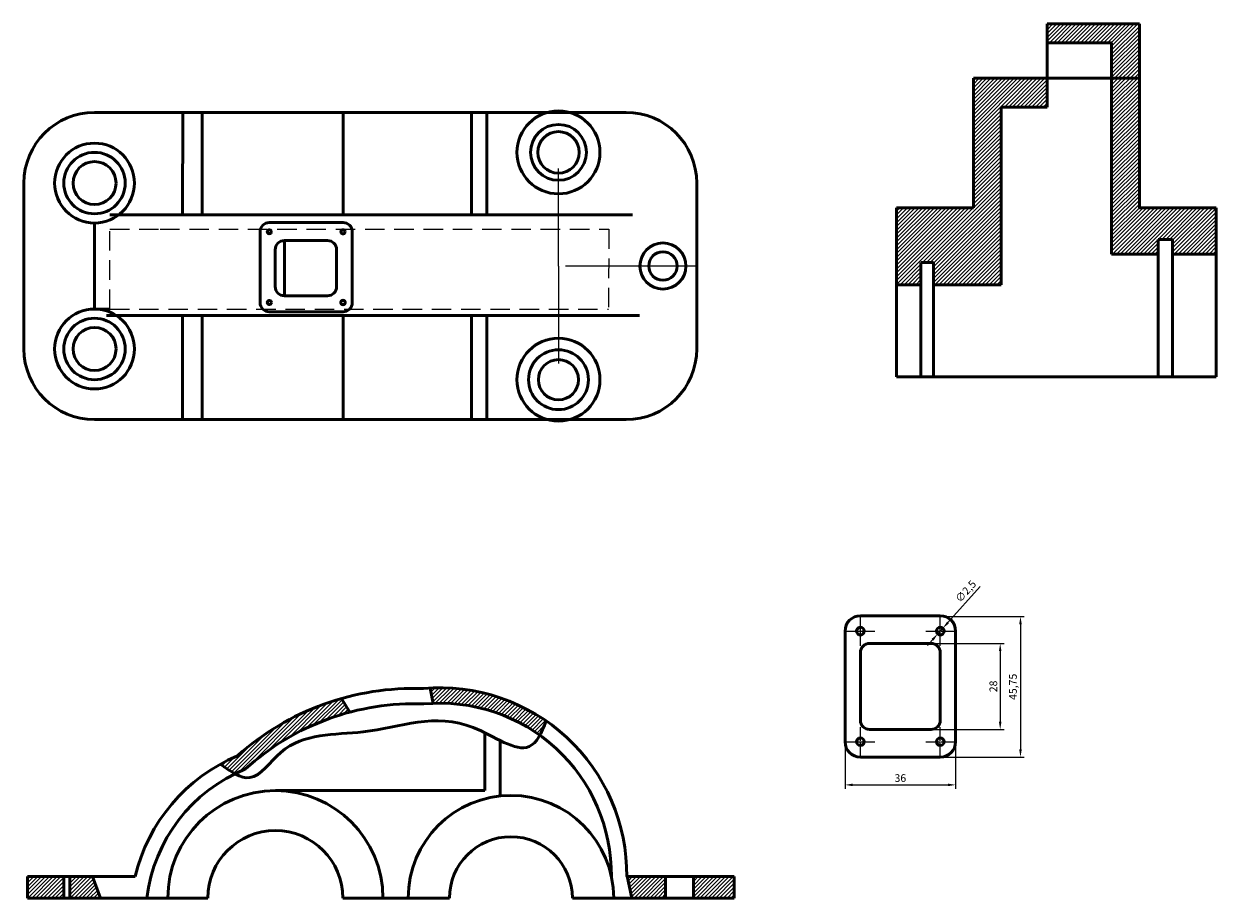
# Model space of a CAD drawing. Units: millimetres. Extents: x 982 to 1370, y 1632 to 1917.
import ezdxf

# ---------------------------------------------------------------- set-up
doc = ezdxf.new("R2010")
doc.units = ezdxf.units.MM
doc.linetypes.add('CENTER', pattern=[50.800000000000004, 31.75, -6.349999999999999, 6.349999999999999, -6.349999999999999])
doc.linetypes.add('HIDDEN', pattern=[9.524999999999999, 6.349999999999999, -3.174999999999999])
for name, color, linetype, lineweight in [('M-CNTR', 1, 'CENTER', 18), ('M-DIMS', 2, 'Continuous', 25), ('M-HATC', 8, 'Continuous', 18), ('M-HIDN', 6, 'HIDDEN', 25), ('M-OUTL', 7, 'Continuous', 50)]:
    doc.layers.add(name, color=color, linetype=linetype, lineweight=lineweight)
doc.styles.get("Standard").update_dxf_attribs({"font": 'arial.ttf'})
doc.dimstyles.new('ISO-25', dxfattribs={"dimtxt": 2.5, "dimasz": 2.5, "dimexe": 1.25, "dimexo": 0.625, "dimtad": 1, "dimtxsty": 'Standard', "dimcen": 2.5, "dimadec": 0, "dimazin": 0, "dimtfac": 1, "dimtmove": 0, "dimatfit": 3, "dimfxl": 1, "dimarcsym": 0})
pattern_1 = [(45, (0, 0), (-0.6286179284748407, 0.6286179284748407), [])]

# ---------------------------------------------------------------- blocks, each defined once
blk = doc.blocks.new('*U1')
at = {"layer": 'M-CNTR', "color": 0, "transparency": 16777216}
for p, q in [((0, 0.25), (0, 4.75)), ((-4.75, 0), (-0.25, 0)), ((0.25, 0), (4.75, 0)), ((0, -4.75), (0, -0.25))]:
    blk.add_line(p, q, dxfattribs=at)
at = {"layer": 'M-CNTR', "color": 0, "linetype": 'Continuous', "transparency": 16777216}
for p, q in [((-0.125, 0), (0.125, 0)), ((0, -0.125), (0, 0.125))]:
    blk.add_line(p, q, dxfattribs=at)
blk = doc.blocks.new('*U2')
at = {"layer": 'M-CNTR', "color": 0, "transparency": 16777216}
for p, q in [((0, 0.25), (0, 4.75)), ((-4.75, 0), (-0.25, 0)), ((0.25, 0), (4.75, 0)), ((0, -4.75), (0, -0.25))]:
    blk.add_line(p, q, dxfattribs=at)
at = {"layer": 'M-CNTR', "color": 0, "linetype": 'Continuous', "transparency": 16777216}
for p, q in [((-0.125, 0), (0.125, 0)), ((0, -0.125), (0, 0.125))]:
    blk.add_line(p, q, dxfattribs=at)
blk = doc.blocks.new('*U3')
at = {"layer": 'M-CNTR', "color": 0, "transparency": 16777216}
for p, q in [((0, 0.25), (0, 4.75)), ((-4.75, 0), (-0.25, 0)), ((0.25, 0), (4.75, 0)), ((0, -4.75), (0, -0.25))]:
    blk.add_line(p, q, dxfattribs=at)
at = {"layer": 'M-CNTR', "color": 0, "linetype": 'Continuous', "transparency": 16777216}
for p, q in [((-0.125, 0), (0.125, 0)), ((0, -0.125), (0, 0.125))]:
    blk.add_line(p, q, dxfattribs=at)
blk = doc.blocks.new('*U4')
at = {"layer": 'M-CNTR', "color": 0, "transparency": 16777216}
for p, q in [((0, 0.25), (0, 4.75)), ((-4.75, 0), (-0.25, 0)), ((0.25, 0), (4.75, 0)), ((0, -4.75), (0, -0.25))]:
    blk.add_line(p, q, dxfattribs=at)
at = {"layer": 'M-CNTR', "color": 0, "linetype": 'Continuous', "transparency": 16777216}
for p, q in [((-0.125, 0), (0.125, 0)), ((0, -0.125), (0, 0.125))]:
    blk.add_line(p, q, dxfattribs=at)
blk = doc.blocks.new('*D5')
at = {"layer": 'Defpoints', "color": 0, "transparency": 16777216}
for p in [(1249.511989077973, 1683.208601525211), (1285.511989077973, 1683.208601525211), (1285.511989077973, 1669.151294933958)]:
    blk.add_point(p, dxfattribs=at)
at = {"layer": 'M-DIMS', "color": 0, "lineweight": -2, "transparency": 16777216}
for p, q in [((1249.511989077973, 1682.583601525211), (1249.511989077973, 1667.901294933958)), ((1285.511989077973, 1682.583601525211), (1285.511989077973, 1667.901294933958)), ((1252.011989077973, 1669.151294933958), (1283.011989077973, 1669.151294933958))]:
    blk.add_line(p, q, dxfattribs=at)
at = {"layer": 'M-DIMS', "color": 0, "transparency": 16777216}
for points in [[(1252.011989077973, 1669.567961600625), (1252.011989077973, 1668.734628267292), (1249.511989077973, 1669.151294933958)], [(1283.011989077973, 1669.567961600625), (1283.011989077973, 1668.734628267292), (1285.511989077973, 1669.151294933958)]]:
    blk.add_solid(points, dxfattribs=at)
at = {"layer": 'M-DIMS', "color": 0, "transparency": 16777216, "insert": (1267.511989077973, 1671.053580063563), "char_height": 2.5, "attachment_point": 5}
blk.add_mtext('36', dxfattribs=at)
blk = doc.blocks.new('*D6')
at = {"layer": 'Defpoints', "color": 0, "transparency": 16777216}
for p in [(1280.511989077974, 1723.958601525212), (1280.511989077974, 1678.208601525212), (1306.611679596875, 1678.208601525212)]:
    blk.add_point(p, dxfattribs=at)
at = {"layer": 'M-DIMS', "color": 0, "lineweight": -2, "transparency": 16777216}
for p, q in [((1281.136989077974, 1723.958601525212), (1307.861679596875, 1723.958601525212)), ((1306.611679596875, 1721.458601525213), (1306.611679596875, 1680.708601525212)), ((1281.136989077974, 1678.208601525212), (1307.861679596875, 1678.208601525212))]:
    blk.add_line(p, q, dxfattribs=at)
at = {"layer": 'M-DIMS', "color": 0, "transparency": 16777216}
for points in [[(1306.195012930208, 1721.458601525213), (1307.028346263542, 1721.458601525213), (1306.611679596875, 1723.958601525212)], [(1306.195012930208, 1680.708601525212), (1307.028346263542, 1680.708601525212), (1306.611679596875, 1678.208601525212)]]:
    blk.add_solid(points, dxfattribs=at)
at = {"layer": 'M-DIMS', "color": 0, "transparency": 16777216, "insert": (1304.489408109836, 1701.083601525211), "char_height": 2.5, "attachment_point": 5, "rotation": 90}
blk.add_mtext('45,75', dxfattribs=at)
blk = doc.blocks.new('*D7')
at = {"layer": 'Defpoints', "color": 0, "transparency": 16777216}
for p in [(1277.511989077974, 1715.208601525213), (1277.511989077974, 1687.208601525212), (1300.009759810087, 1687.208601525212)]:
    blk.add_point(p, dxfattribs=at)
at = {"layer": 'M-DIMS', "color": 0, "lineweight": -2, "transparency": 16777216}
for p, q in [((1278.136989077974, 1715.208601525213), (1301.259759810087, 1715.208601525213)), ((1300.009759810087, 1712.708601525212), (1300.009759810087, 1689.708601525212)), ((1278.136989077974, 1687.208601525212), (1301.259759810087, 1687.208601525212))]:
    blk.add_line(p, q, dxfattribs=at)
at = {"layer": 'M-DIMS', "color": 0, "transparency": 16777216}
for points in [[(1299.59309314342, 1712.708601525212), (1300.426426476754, 1712.708601525212), (1300.009759810087, 1715.208601525213)], [(1299.59309314342, 1689.708601525212), (1300.426426476754, 1689.708601525212), (1300.009759810087, 1687.208601525212)]]:
    blk.add_solid(points, dxfattribs=at)
at = {"layer": 'M-DIMS', "color": 0, "transparency": 16777216, "insert": (1298.108327340783, 1701.208601525212), "char_height": 2.5, "attachment_point": 5, "rotation": 90}
blk.add_mtext('28', dxfattribs=at)
blk = doc.blocks.new('*D8')
at = {"layer": 'Defpoints', "color": 0, "transparency": 16777216}
for p in [(1281.346385037726, 1720.139344981997), (1279.677593118221, 1718.277858068427)]:
    blk.add_point(p, dxfattribs=at)
at = {"layer": 'M-DIMS', "color": 0, "lineweight": -2, "transparency": 16777216}
for p, q in [((1293.494623055285, 1733.690337066936), (1283.015176957231, 1722.000831895568)), ((1279.677593118221, 1718.277858068427), (1281.346385037726, 1720.139344981997)), ((1278.008801198716, 1716.416371154856), (1276.34000927921, 1714.554884241286))]:
    blk.add_line(p, q, dxfattribs=at)
at = {"layer": 'M-DIMS', "color": 0, "transparency": 16777216}
for points in [[(1282.704929138303, 1722.278963882152), (1283.32542477616, 1721.722699908983), (1281.346385037726, 1720.139344981997)], [(1277.698553379787, 1716.69450314144), (1278.319049017644, 1716.138239168272), (1279.677593118221, 1718.277858068427)]]:
    blk.add_solid(points, dxfattribs=at)
at = {"layer": 'M-DIMS', "color": 0, "transparency": 16777216, "insert": (1289.029728391543, 1731.958212710914), "char_height": 2.5, "attachment_point": 5, "rotation": 48.12430414894632}
blk.add_mtext('∅2,5', dxfattribs=at)

msp = doc.modelspace()

# ---------------------------------------------------------------- hatches: boundary and pattern name
at = {"layer": 'M-HATC'}
h = msp.add_hatch(dxfattribs=at)
h.set_pattern_fill('ANSI31', color=256, scale=0.28)
h.set_pattern_definition(pattern_1)
h.paths.add_polyline_path([(1300.29876673081, 1889.791887260162), (1315.29876673081, 1889.791887260162), (1315.29876673081, 1899.183957242303), (1291.29876673081, 1899.183957242303), (1291.29876673081, 1856.97244571802), (1266.29876673081, 1856.97244571802), (1266.29876673081, 1831.97244571802), (1274.206576974626, 1831.97244571802), (1274.206576974626, 1839.244321779904), (1278.280369147082, 1839.244321779905), (1278.280369147082, 1831.97244571802), (1300.29876673081, 1831.97244571802)])
h.paths.add_polyline_path([(1370.29876673081, 1856.97244571802), (1345.29876673081, 1856.97244571802), (1345.29876673081, 1899.183957242303), (1336.285268659707, 1899.183957242303), (1336.285268659707, 1841.97244571802), (1351.382184464795, 1841.97244571802), (1351.382184464795, 1846.706406237832), (1356.134930561908, 1846.706406237832), (1356.134930561908, 1841.97244571802), (1370.29876673081, 1841.97244571802)])
h.paths.add_polyline_path([(1345.29876673081, 1916.899596030982), (1340.29876673081, 1916.899596030982), (1315.29876673081, 1916.899596030982), (1315.29876673081, 1910.726026523388), (1336.285268659707, 1910.726026523388), (1336.285268659707, 1899.183957242303), (1345.29876673081, 1899.183957242303)])
h = msp.add_hatch(dxfattribs=at)
h.set_pattern_fill('ANSI31', color=256, scale=0.28)
h.set_pattern_definition(pattern_1)
h.paths.add_polyline_path([(995.2535490241661, 1639.282014954298), (983.4732738171352, 1639.282014954298), (983.4732738171352, 1632.282014954298), (995.2535490241661, 1632.282014954298)])
h.paths.add_polyline_path([(1004.648487103659, 1639.282014954298), (997.2535490241662, 1639.282014954298), (997.2535490241662, 1632.282014954298), (1007.250709303537, 1632.282014954298)])
edge = h.paths.add_edge_path()
edge.add_line((1088.387454769102, 1692.837831887581), (1085.605211651708, 1697.258198737764))
edge.add_arc((1109.271975537356, 1614.115057323262), 86.44592342667784, 105.8890469631471, 131.7276792270625)
edge.add_arc((1074.062003103345, 1626.025891843346), 57.14745509284148, 112.9982183834284, 119.206106940538)
edge.add_spline(control_points=[(1046.176748216584, 1675.908195153124), (1047.783063834055, 1674.759506472575), (1049.389379451526, 1673.610817792025), (1050.94946138008, 1672.771666922494)], knot_values=[0, 0, 0, 0, 5.081182044010842, 5.081182044010842, 5.081182044010842, 5.081182044010842], degree=3, periodic=0)
edge.add_arc((1074.062003103346, 1626.025891843347), 52.14745509284142, 112.09848204372611, 116.30920051008201, ccw=False)
edge.add_arc((1109.271975537356, 1614.115057323262), 81.44592342667777, 104.8578574495586, 132.313036151602, ccw=False)
edge = h.paths.add_edge_path()
edge.add_line((1114.536751154887, 1700.664583068479), (1115.499488170572, 1695.703224651357))
edge.add_arc((1117.676663324449, 1639.945484012596), 55.80023058007832, 54.3761729250636, 92.23609505560682, ccw=False)
edge.add_spline(control_points=[(1150.178124588469, 1685.303181799117), (1150.925335073614, 1686.661176424872), (1151.580506534144, 1688.273325651683), (1152.195395815112, 1689.996709230653)], knot_values=[112.2880017170733, 112.2880017170733, 112.2880017170733, 112.2880017170733, 116.9515328515951, 116.9515328515951, 116.9515328515951, 116.9515328515951], degree=3, periodic=0)
edge.add_arc((1117.676663324449, 1639.945484012596), 60.80023058007828, 55.40721006559874, 92.96024829593541)
h.paths.add_polyline_path([(1191.134183879782, 1639.282014954298), (1178.620543520746, 1639.282014954298), (1180.136133887702, 1632.282014954298), (1191.134183879781, 1632.282014954298)])
h.paths.add_polyline_path([(1213.473273817135, 1639.282014954298), (1200.175070862797, 1639.282014954298), (1200.175070862797, 1632.282014954298), (1213.473273817135, 1632.282014954298)])

# ---------------------------------------------------------------- linework, layer by layer
at = {"layer": 'M-CNTR'}
for p, q in [((1156.251070972097, 1838.057992080775), (1156.251070972097, 1875.057992080776)), ((1190.251070972097, 1838.057992080775), (1156.251070972097, 1838.057992080775)), ((1156.251070972097, 1838.057992080775), (1156.251070972097, 1801.057992080776)), ((1201.251070972097, 1838.057992080775), (1190.251070972097, 1838.057992080775))]:
    msp.add_line(p, q, dxfattribs=at)
at = {"layer": 'M-HIDN'}
for p, q in [((1010.251070972097, 1824.057992080776), (1010.251070972097, 1850.036021916558)), ((1010.251070972097, 1850.036021916558), (1026.612848150797, 1850.036021916558)), ((1026.612848150797, 1850.036021916558), (1172.670257073025, 1850.036021916558)), ((1172.670257073025, 1850.036021916558), (1172.528142112141, 1824.057992080776)), ((1010.251070972097, 1824.057992080776), (1172.528142112141, 1824.057992080776))]:
    msp.add_line(p, q, dxfattribs=at)
at = {"layer": 'M-OUTL'}
for p, q in [((1315.29876673081, 1889.791887260162), (1315.29876673081, 1916.899596030982)), ((1315.29876673081, 1916.899596030982), (1340.29876673081, 1916.899596030982)), ((1340.29876673081, 1916.899596030982), (1345.29876673081, 1916.899596030982)), ((1345.29876673081, 1916.899596030982), (1345.29876673081, 1899.183957242303)), ((1336.285268659707, 1910.726026523388), (1315.29876673081, 1910.726026523388)), ((1336.285268659707, 1841.97244571802), (1336.285268659707, 1910.726026523388)), ((1291.29876673081, 1856.97244571802), (1291.29876673081, 1899.183957242303)), ((1291.29876673081, 1899.183957242303), (1345.29876673081, 1899.183957242303)), ((1345.29876673081, 1856.97244571802), (1345.29876673081, 1899.183957242303)), ((1005.251070972097, 1888.057992080776), (1178.251070972097, 1888.057992080776)), ((1034.029285878291, 1888.057992080776), (1033.904053084971, 1854.694341917483)), ((1040.294262971387, 1888.057992080776), (1040.294262971387, 1854.694341917483)), ((1086.162194136173, 1888.057992080776), (1086.162194136173, 1854.694341917483)), ((1127.916033374389, 1888.057992080776), (1127.916033374389, 1854.694341917483)), ((1132.916033374389, 1854.694341917483), (1132.916033374389, 1888.057992080776)), ((1300.29876673081, 1831.97244571802), (1300.29876673081, 1889.791887260162)), ((1300.29876673081, 1889.791887260162), (1315.29876673081, 1889.791887260162)), ((982.2510709720972, 1811.057992080776), (982.2510709720972, 1865.057992080776)), ((1201.251070972097, 1811.057992080776), (1201.251070972097, 1865.057992080776)), ((1266.29876673081, 1801.97244571802), (1266.29876673081, 1856.97244571802)), ((1266.29876673081, 1856.97244571802), (1291.29876673081, 1856.97244571802)), ((1266.29876673081, 1856.97244571802), (1266.29876673081, 1831.97244571802)), ((1370.29876673081, 1856.97244571802), (1345.29876673081, 1856.97244571802)), ((1370.29876673081, 1801.97244571802), (1370.29876673081, 1856.97244571802)), ((1370.29876673081, 1856.97244571802), (1370.29876673081, 1841.97244571802)), ((1005.251070972097, 1852.057992080776), (1005.251070972097, 1824.057992080776)), ((1010.252314597974, 1854.694341917483), (1180.329749461996, 1854.694341917483)), ((1062.143259161312, 1852.211589826624), (1086.143259161312, 1852.211589826624)), ((1059.143259161312, 1849.211589826624), (1059.143259161312, 1826.179334016416)), ((1089.143259161312, 1826.179334016416), (1089.143259161312, 1849.211589826624)), ((1064.050993755085, 1831.375096835255), (1064.050993755085, 1843.375096835255)), ((1067.050993755085, 1846.375096835255), (1081.050993755085, 1846.375096835255)), ((1067.050993755085, 1846.375096835255), (1067.050993755085, 1828.375096835255)), ((1084.050993755085, 1843.375096835255), (1084.050993755085, 1831.375096835255)), ((1351.382184464795, 1846.706406237832), (1351.382184464795, 1801.97244571802)), ((1351.382184464795, 1846.706406237832), (1356.134930561908, 1846.706406237832)), ((1356.134930561908, 1801.97244571802), (1356.134930561908, 1846.706406237832)), ((1351.382184464795, 1841.97244571802), (1336.285268659707, 1841.97244571802)), ((1370.29876673081, 1841.97244571802), (1356.134930561908, 1841.97244571802)), ((1274.206576974626, 1839.244321779904), (1274.206576974626, 1801.97244571802)), ((1274.206576974626, 1839.244321779904), (1278.280369147082, 1839.244321779905)), ((1278.280369147082, 1801.97244571802), (1278.280369147082, 1839.244321779905)), ((1266.29876673081, 1831.97244571802), (1274.206576974626, 1831.97244571802)), ((1278.280369147082, 1831.97244571802), (1300.29876673081, 1831.97244571802)), ((1081.050993755085, 1828.375096835255), (1067.050993755085, 1828.375096835255)), ((1005.251070972097, 1824.057992080776), (1010.251070972097, 1824.057992080776)), ((1009.203594559912, 1821.924287656346), (1182.625737453978, 1821.924287656346)), ((1033.904053084971, 1821.924287656345), (1033.904053084971, 1788.057992080776)), ((1040.294262971387, 1821.924287656346), (1040.294262971387, 1788.057992080776)), ((1062.143259161312, 1823.179334016416), (1086.143259161312, 1823.179334016416)), ((1086.162194136173, 1821.924287656346), (1086.162194136173, 1788.057992080776)), ((1127.916033374389, 1821.924287656345), (1127.916033374389, 1788.057992080776)), ((1132.916033374389, 1821.924287656345), (1132.916033374389, 1788.057992080776)), ((1266.29876673081, 1801.97244571802), (1370.29876673081, 1801.97244571802)), ((1005.251070972097, 1788.057992080776), (1178.251070972097, 1788.057992080776)), ((1254.511989077973, 1724.208601525212), (1280.511989077973, 1724.208601525212)), ((1249.511989077973, 1683.208601525211), (1249.511989077973, 1719.208601525211)), ((1285.511989077973, 1719.208601525211), (1285.511989077973, 1683.208601525211)), ((1257.511989077973, 1715.208601525211), (1277.511989077973, 1715.208601525211)), ((1254.511989077973, 1701.208601525211), (1254.511989077973, 1712.208601525211)), ((1280.511989077973, 1712.208601525211), (1280.511989077973, 1690.208601525212)), ((1114.536751154887, 1700.664583068479), (1115.499488170572, 1695.703224651357)), ((1254.511989077973, 1690.208601525212), (1254.511989077973, 1701.208601525211)), ((1085.605211651708, 1697.258198737765), (1088.387454769102, 1692.837831887581)), ((1132.322723132545, 1667.282014954298), (1132.322723132545, 1686.107194496415)), ((1277.511989077973, 1687.208601525211), (1257.511989077973, 1687.208601525211)), ((1137.322723132545, 1683.568690464403), (1137.322723132545, 1665.554162394855)), ((1280.511989077973, 1678.208601525211), (1254.511989077973, 1678.208601525211)), ((1064.107042838392, 1667.282014954298), (1132.322723132545, 1667.282014954298)), ((983.4732738171352, 1632.282014954298), (983.4732738171352, 1639.282014954298)), ((983.4732738171352, 1639.282014954298), (1018.473273817135, 1639.282014954298)), ((995.2535490241661, 1639.282014954298), (995.2535490241661, 1632.282014954298)), ((997.2535490241662, 1632.282014954298), (997.2535490241662, 1639.282014954298)), ((1004.648487103659, 1639.282014954298), (1007.250709303538, 1632.282014954298)), ((1213.473273817135, 1639.282014954298), (1178.473273817135, 1639.282014954298)), ((1178.476893904527, 1639.945484012596), (1180.136133887702, 1632.282014954298)), ((1191.134183879782, 1639.282014954298), (1191.134183879781, 1632.282014954298)), ((1200.175070862797, 1632.282014954298), (1200.175070862797, 1639.282014954298)), ((1213.473273817135, 1632.282014954298), (1213.473273817135, 1639.282014954298)), ((983.4732738171352, 1632.282014954298), (1042.107042838392, 1632.282014954298)), ((1086.107042838392, 1632.282014954298), (1107.326722726267, 1632.282014954298)), ((1107.326722726267, 1632.282014954298), (1120.777779675505, 1632.282014954298)), ((1160.777779675505, 1632.282014954298), (1174.228836624744, 1632.282014954298)), ((1174.228836624744, 1632.282014954298), (1213.473273817135, 1632.282014954298))]:
    msp.add_line(p, q, dxfattribs=at)
for centre, radius in [((1156.251070972097, 1875.057992080776), 13.5), ((1156.251070972097, 1875.057992080776), 9.083792335562066), ((1156.251070972097, 1875.057992080776), 6.750000000000017), ((1005.251070972097, 1865.057992080776), 13), ((1005.251070972097, 1865.057992080776), 10), ((1005.251070972097, 1865.057992080776), 7), ((1062.143259161312, 1849.211589826624), 0.6479663108375462), ((1086.143259161312, 1849.211589826624), 0.6787768738613523), ((1190.251070972097, 1838.057992080775), 7.5), ((1190.251070972097, 1838.057992080775), 7.5), ((1190.251070972097, 1838.057992080775), 4.627422957195904), ((1005.251070972097, 1811.057992080776), 13), ((1062.143259161312, 1826.179334016416), 0.6787768738613523), ((1086.143259161312, 1826.179334016416), 0.7312833828641488), ((1005.251070972097, 1811.057992080776), 10), ((1005.251070972097, 1811.057992080776), 7), ((1156.251070972097, 1801.057992080776), 13.5), ((1156.251070972097, 1801.057992080776), 9.73825588175896), ((1156.251070972097, 1801.057992080776), 6.532587590030743), ((1254.511989077973, 1719.208601525211), 1.25), ((1280.511989077973, 1719.208601525211), 1.25), ((1254.511989077973, 1683.208601525211), 1.25), ((1280.511989077973, 1683.208601525211), 1.25)]:
    msp.add_circle(centre, radius, dxfattribs=at)
for centre, radius, start, end in [((1005.251070972097, 1865.057992080776), 23, 90, 180), ((1178.251070972097, 1865.057992080776), 23, 0, 90), ((1062.143259161312, 1849.211589826624), 3, 90, 180), ((1086.143259161312, 1849.211589826624), 3, 359.9999999999996, 90), ((1067.050993755085, 1843.375096835255), 3, 90, 180), ((1081.050993755085, 1843.375096835255), 3, 0, 90), ((1067.050993755085, 1831.375096835255), 3, 180, 270), ((1081.050993755085, 1831.375096835255), 3, 270, 0), ((1062.143259161312, 1826.179334016416), 3, 180, 270), ((1086.143259161312, 1826.179334016416), 3, 270, 359.9999999999995), ((1005.251070972097, 1811.057992080776), 23, 180, 270), ((1178.251070972097, 1811.057992080776), 23, 270, 0), ((1254.511989077973, 1719.208601525211), 5, 90, 180), ((1280.511989077973, 1719.208601525211), 5, 0, 90), ((1257.511989077973, 1712.208601525211), 3, 90, 180), ((1277.511989077973, 1712.208601525211), 3, 0, 90), ((1109.271975537356, 1614.115057323262), 86.44592342667784, 87.99040007700376, 131.7276792270625), ((1117.676663324449, 1639.945484012596), 60.80023058007828, 359.3747600791531, 95.07019799439956), ((1109.271975537356, 1614.115057323262), 81.44592342667784, 87.77134775830568, 132.3130361515951), ((1117.676663324449, 1639.945484012596), 55.80023058007828, 359.3880265313779, 95.3857598229008), ((1257.511989077973, 1690.208601525212), 3, 180, 270), ((1277.511989077973, 1690.208601525212), 3, 270, 0), ((1254.511989077973, 1683.208601525211), 5, 180, 270), ((1280.511989077973, 1683.208601525211), 5, 270, 0), ((1074.062003103346, 1626.025891843347), 57.14745509284148, 112.9982183834288, 166.5873017965039), ((1074.062003103346, 1626.025891843347), 52.14745509284148, 112.0984820437266, 173.1096366337904), ((1064.107042838392, 1632.282014954298), 35, 0, 180), ((1140.777779675505, 1632.282014954298), 33.45105694923859, 0, 180), ((1064.107042838392, 1632.282014954298), 22, 0, 180), ((1140.777779675505, 1632.282014954298), 20, 0, 180)]:
    msp.add_arc(centre, radius, start, end, dxfattribs=at)
msp.add_open_spline([(1046.176748216584, 1675.908195153124), (1049.507842932328, 1673.526103643712), (1056.96131843453, 1668.196065855988), (1068.671375052202, 1686.644958170573), (1096.251597707593, 1684.141895742433), (1122.014518166959, 1695.401452051044), (1146.265477752429, 1676.650571966315), (1150.793560932861, 1686.067710480346), (1152.195395815112, 1689.996709230653)], degree=3, knots=[0, 0, 0, 0, 10.53709400098201, 23.57722571787429, 51.23048866659805, 87.0716660520638, 106.3195364561623, 116.9515328515951, 116.9515328515951, 116.9515328515951, 116.9515328515951], dxfattribs=at)

# ---------------------------------------------------------------- block references
at = {"layer": 'M-CNTR'}
for name, p in [('*U1', (1254.511989077973, 1719.208601525211)), ('*U2', (1280.511989077973, 1719.208601525211)), ('*U4', (1254.511989077973, 1683.208601525211)), ('*U3', (1280.511989077973, 1683.208601525211))]:
    msp.add_blockref(name, p, dxfattribs=at)

# ---------------------------------------------------------------- dimensions: what is measured, and where the dimension line sits
at = {"layer": 'M-DIMS'}
dim = msp.add_diameter_dim_2p(p1=(1279.677593118221, 1718.277858068427), p2=(1281.346385037726, 1720.139344981997), dimstyle='ISO-25', override={"dimclrd": 0, "dimclre": 0, "dimclrt": 0}, dxfattribs=at)
dim.commit()
dim.dimension.update_dxf_attribs({"geometry": '*D8', "text_midpoint": (1290.644244497004, 1730.510825994917), "dimtype": 163})
for base, p1, p2, picture, middle in [((1306.611679596875, 1678.208601525212), (1280.511989077973, 1723.958601525211), (1280.511989077973, 1678.208601525211), '*D6', (1304.489408109836, 1701.083601525211)), ((1300.009759810087, 1687.208601525212), (1277.511989077973, 1715.208601525211), (1277.511989077973, 1687.208601525211), '*D7', (1298.108327340783, 1701.208601525212))]:
    dim = msp.add_linear_dim(base=base, p1=p1, p2=p2, angle=90, dimstyle='ISO-25', override={"dimclrd": 0, "dimclre": 0, "dimclrt": 0}, dxfattribs=at)
    dim.commit()
    dim.dimension.update_dxf_attribs({"geometry": picture, "text_midpoint": middle})
dim = msp.add_linear_dim(base=(1285.511989077973, 1669.151294933958), p1=(1249.511989077973, 1683.208601525211), p2=(1285.511989077973, 1683.208601525211), dimstyle='ISO-25', override={"dimclrd": 0, "dimclre": 0, "dimclrt": 0}, dxfattribs=at)
dim.commit()
dim.dimension.update_dxf_attribs({"geometry": '*D5', "text_midpoint": (1267.511989077973, 1671.053580063563)})

doc.saveas('drawing.dxf')
